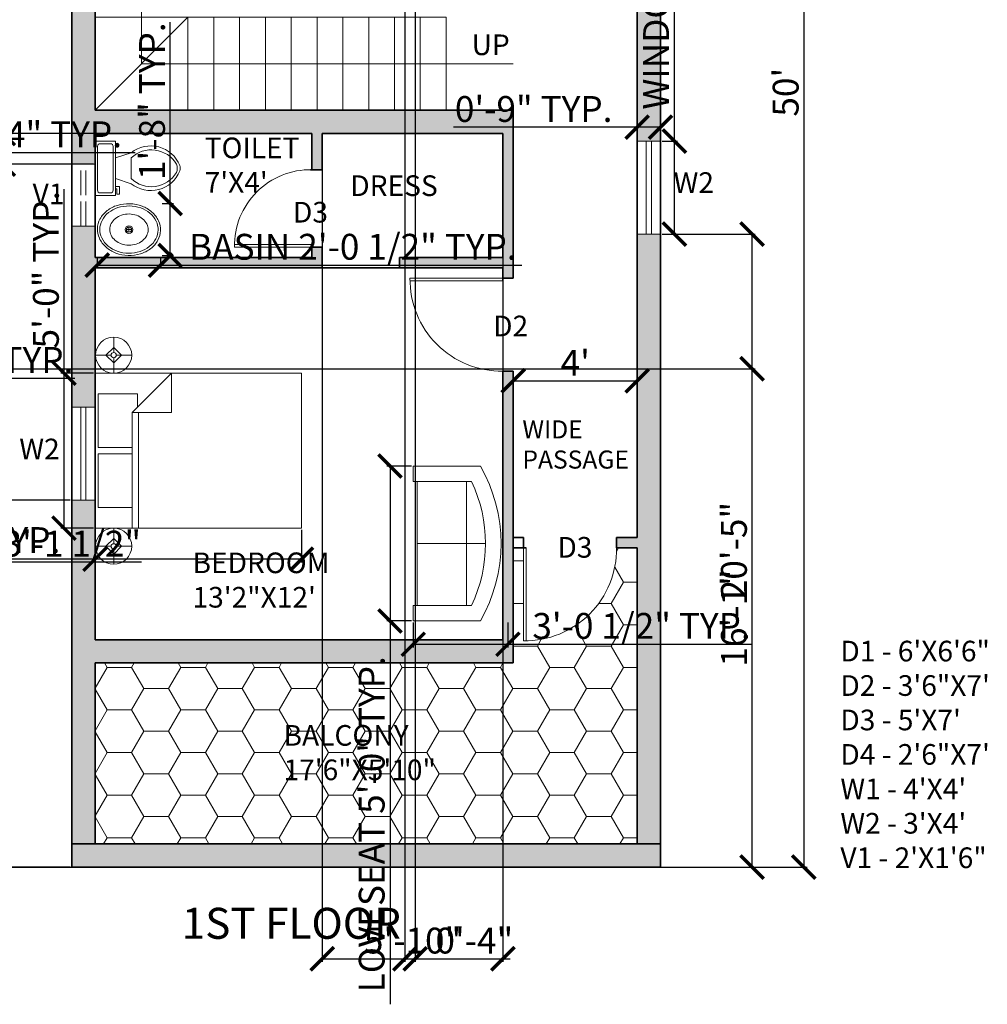
# Model space of a CAD drawing. Units: inches. Extents: x 2570 to 3313, y 1387 to 2106.
# Tile 4 of 5: x 2938 to 3313, y 1387 to 1769. Entities that reach past the tile are written whole.
import ezdxf

# ---------------------------------------------------------------- set-up
doc = ezdxf.new("R2010")
doc.units = ezdxf.units.IN
doc.linetypes.add('ACAD_ISO02W100', pattern=[15, 12, -3])
for name, color, linetype, lineweight in [('A-ANNO-DIMS', 7, 'Continuous', 18), ('A-ANNO-SYMB', 13, 'Continuous', 13), ('bed', 221, 'Continuous', 18), ('DOORS', 195, 'Continuous', 18), ('furniture', 11, 'Continuous', 18), ('P-FIXT', 8, 'Continuous', 18), ('STAIRS', 13, 'Continuous', 18), ('VENTILATORS', 143, 'ACAD_ISO02W100', 18), ('WALLS', 20, 'Continuous', 35), ('WINDOWS', 15, 'Continuous', 18)]:
    doc.layers.add(name, color=color, linetype=linetype, lineweight=lineweight)
for name, color, linetype, lineweight, true_color in [('A-ANNO-TEXT', 143, 'Continuous', 18, 0x7aafdf), ('A-ANNO-TITL', 52, 'Continuous', 25, 0xc8c92d), ('A-AREA-IDEN', 143, 'Continuous', 18, 0x7aafdf), ('A-FLOR-PATT', 254, 'Continuous', 13, 0xcecce6), ('A-WALL-PATT', 30, 'Continuous', 13, 0xf26722)]:
    doc.layers.add(name, color=color, linetype=linetype, lineweight=lineweight, true_color=true_color)
doc.styles.get("Standard").update_dxf_attribs({"font": 'arial.ttf'})
doc.dimstyles.new('ISO-25', dxfattribs={"dimtxt": 10, "dimasz": 9, "dimexe": 1.25, "dimexo": 0.625, "dimtad": 1, "dimdec": 0, "dimlunit": 3, "dimtxsty": 'Standard', "dimblk": 'ARCHTICK', "dimcen": 2.5, "dimadec": 0, "dimazin": 0, "dimtfac": 1, "dimtdec": 0, "dimtmove": 0, "dimatfit": 3, "dimfxl": 1, "dimarcsym": 0})

# ---------------------------------------------------------------- blocks, each defined once
blk = doc.blocks.new('Lamp - Table')
for p, q in [((0, 7), (0, 1)), ((-1, 0), (-7, 0)), ((0, 3), (-3, 0)), ((-3, 0), (0, -3)), ((3, 0), (0, 3)), ((0, -3), (3, 0)), ((1, 0), (7, 0)), ((0, -1), (0, -7))]:
    blk.add_line(p, q)
for radius in [7, 1]:
    blk.add_circle((0, 0), radius)
blk = doc.blocks.new('Bed - Queen')
for p, q in [((0, -80.00003), (0, 0)), ((0, 0), (59.99999, 0)), ((59.99999, 0), (59.99999, -80.00003)), ((7.99999, -1.2), (28.79998, -1.2)), ((7.99999, -14.4), (7.99999, -1.2)), ((28.79998, -1.2), (28.79998, -14.4)), ((31.19999, -1.2), (51.99999, -1.2)), ((31.19999, -14.4), (31.19999, -1.2)), ((51.99999, -1.2), (51.99999, -16.4)), ((0, -14.4), (44.8, -14.4)), ((59.99999, -29.6), (44.8, -14.4)), ((44.8, -14.4), (44.8, -29.6)), ((44.8, -16.8), (0, -16.8)), ((51.99999, -16.4), (46.79936, -16.4)), ((44.8, -29.6), (59.99999, -29.6)), ((59.99999, -80.00003), (0, -80.00003))]:
    blk.add_line(p, q)
blk = doc.blocks.new('Toilet - top')
for p, q in [((9.5, -6), (9.5, -2)), ((-10, -8.5), (-8, -8.5)), ((-10, -9.5), (-10, -8.5)), ((-7, -9.5), (-10, -9.5)), ((-8, -8.5), (-8, -8)), ((-7, -8), (-7, -9.5)), ((-4, -8), (-6, -14)), ((4, -8), (6, -14)), ((4, -14), (-4, -14))]:
    blk.add_line(p, q)
blk.add_lwpolyline([(10.5, -8), (10.5, 0), (-10.5, 0), (-10.5, -8)], close=True)
for points in [[(-9.5, -2), (-9.5, -6)], [(8.5, -1), (-8.5, -1)], [(-8.5, -7), (8.5, -7)]]:
    blk.add_lwpolyline(points)
for centre, radius, start, end in [((-8.62, -1.88), 0.884, 81.8699, 188.1301), ((8.62, -1.88), 0.884, 351.8699, 98.1301), ((-8.62, -6.12), 0.884, 171.8699, 278.1301), ((8.62, -6.12), 0.884, 261.8699, 8.1301), ((3.52, -21.58), 12.17, 141.4691, 247.9714), ((4.2, -21.82), 11.33, 136.3677, 238.9468), ((-3.52, -21.58), 12.17, 292.0284, 38.5307), ((-4.2, -21.82), 11.33, 301.053, 43.6321), ((0, -27.88), 4, 245.7318, 294.2682), ((0, -29), 4, 254.8605, 285.1395)]:
    blk.add_arc(centre, radius, start, end)
blk = doc.blocks.new('Sofa - Roundback Loveseat 5 ft.')
for p, q in [((0, -32.44198), (0, -5.99998)), ((-24, -33.99998), (-24, -11.46958)), ((-23.9998, -13.38178), (23.99986, -13.38178)), ((24.00004, -33.99998), (24.00004, -11.46958)), ((-24, -32.44198), (24.00004, -32.44198))]:
    blk.add_line(p, q)
for points in [[(-24, -33.99998), (-30, -33.99998), (-30, -7.99998)], [(30.00004, -7.99998), (30.00004, -33.99998), (24.00004, -33.99998)]]:
    blk.add_lwpolyline(points)
for centre, radius, start, end in [((0, -60.24998), 60.24998, 60.13715, 119.8628), ((0, -61.38438), 55.38444, 64.32083, 115.6792)]:
    blk.add_arc(centre, radius, start, end)
blk = doc.blocks.new('Sink - Oval top')
for p, q in [((-1, 0), (1, 0)), ((0, 1), (0, -1))]:
    blk.add_line(p, q)
for points in [[(-12.23, 0.39, 0.117634), (-11.46, -3.36, 0.104469), (-8.88, -6.8, 0.090016), (-5.08, -9.07, 0.08192), (-0.32, -10.02, 0.08192), (4.49, -9.38, 0.090016), (8.42, -7.36, 0.104469), (11.22, -4.09, 0.117634), (12.23, -0.39, 0.117634), (11.46, 3.36, 0.104469), (8.88, 6.8, 0.090016), (5.08, 9.07, 0.08192), (0.32, 10.02, 0.08192), (-4.49, 9.38, 0.090016), (-8.42, 7.36, 0.104469), (-11.22, 4.09, 0.117634)], [(-11.29, 0.16, 0.118622), (-10.52, -3.25, 0.104678), (-8.07, -6.36, 0.089562), (-4.54, -8.37, 0.081185), (-0.13, -9.15, 0.081185), (4.3, -8.49, 0.089562), (7.89, -6.58, 0.104678), (10.42, -3.55, 0.118622), (11.29, -0.16, 0.118622), (10.52, 3.25, 0.104678), (8.07, 6.36, 0.089562), (4.54, 8.37, 0.081185), (0.13, 9.15, 0.081185), (-4.3, 8.49, 0.089562), (-7.89, 6.58, 0.104678), (-10.42, 3.55, 0.118622)], [(-7.42, 0.08, 0.118283), (-6.91, -2.17, 0.104607), (-5.29, -4.21, 0.089718), (-2.97, -5.53, 0.081436), (-0.07, -6.04, 0.081436), (2.84, -5.59, 0.089718), (5.2, -4.33, 0.104607), (6.86, -2.32, 0.118283), (7.42, -0.08, 0.118283), (6.91, 2.17, 0.104607), (5.29, 4.21, 0.089718), (2.97, 5.53, 0.081436), (0.07, 6.04, 0.081436), (-2.84, 5.59, 0.089718), (-5.2, 4.33, 0.104607), (-6.86, 2.32, 0.118283)]]:
    blk.add_lwpolyline(points, format="xyb", close=True)
for radius in [1.5, 1]:
    blk.add_circle((0, 0), radius)
blk = doc.blocks.new('_ArchTick')
at = {"color": 0, "linetype": 'ByBlock', "const_width": 0.15}
blk.add_lwpolyline([(-0.5, -0.5), (0.5, 0.5)], dxfattribs=at)
blk = doc.blocks.new('*D19')
at = {"layer": 'A-ANNO-DIMS', "color": 0, "lineweight": -2, "transparency": 16777216}
for p, q in [((3186.79, 2040.49), (3242.94, 2040.49)), ((3241.69, 2040.49), (3241.69, 1440.49)), ((3186.79, 1440.49), (3242.94, 1440.49))]:
    blk.add_line(p, q, dxfattribs=at)
at = {"layer": 'Defpoints', "color": 0, "transparency": 16777216}
for p in [(3186.16, 2040.49), (3186.16, 1440.49), (3241.69, 1440.49)]:
    blk.add_point(p, dxfattribs=at)
at = {"layer": 'A-ANNO-DIMS', "color": 0, "lineweight": -2, "transparency": 16777216, "xscale": 9, "yscale": 9, "zscale": 9}
for p, rotation in [((3241.69, 2040.49), 90), ((3241.69, 1440.49), 270)]:
    blk.add_blockref('_ArchTick', p, dxfattribs=dict(at, rotation=rotation))
at = {"layer": 'A-ANNO-DIMS', "color": 0, "transparency": 16777216, "insert": (3235.96, 1740.49), "char_height": 10, "attachment_point": 5, "rotation": 90}
blk.add_mtext("50'", dxfattribs=at)
blk = doc.blocks.new('*D23')
at = {"layer": 'A-ANNO-DIMS', "color": 0, "lineweight": -2, "transparency": 16777216}
for p, q in [((3129.16, 1631.86), (3129.16, 1627.51)), ((3177.16, 1631.86), (3177.16, 1627.51)), ((3129.16, 1628.76), (3177.16, 1628.76))]:
    blk.add_line(p, q, dxfattribs=at)
at = {"layer": 'Defpoints', "color": 0, "transparency": 16777216}
for p in [(3129.16, 1632.49), (3177.16, 1632.49), (3177.16, 1628.76)]:
    blk.add_point(p, dxfattribs=at)
at = {"layer": 'A-ANNO-DIMS', "color": 0, "lineweight": -2, "transparency": 16777216, "xscale": 9, "yscale": 9, "zscale": 9, "rotation": 180}
blk.add_blockref('_ArchTick', (3129.16, 1628.76), dxfattribs=at)
at = {"layer": 'A-ANNO-DIMS', "color": 0, "lineweight": -2, "transparency": 16777216, "xscale": 9, "yscale": 9, "zscale": 9}
blk.add_blockref('_ArchTick', (3177.16, 1628.76), dxfattribs=at)
at = {"layer": 'A-ANNO-DIMS', "color": 0, "transparency": 16777216, "insert": (3153.16, 1634.38), "char_height": 10, "attachment_point": 5}
blk.add_mtext("4'", dxfattribs=at)
blk = doc.blocks.new('DOOR-SWING-30IN')
for p, q in [((0, 0), (-30, 0)), ((0, -1), (-30, -1))]:
    blk.add_line(p, q)
blk.add_arc((-0.5, -0.5), 29.5, 179.029, 270.971)
blk = doc.blocks.new('DOOR-SWING-36IN')
for p, q in [((-1, 0), (-1, 36)), ((0, 0), (0, 36))]:
    blk.add_line(p, q)
blk.add_arc((-0.5, 0.5), 35.5, 89.1931, 180.8069)
blk = doc.blocks.new('WIN-36IN')
for p, q in [((-36, 0), (-36, 9)), ((0, 0), (0, 9)), ((-36, 5.5), (0, 5.5)), ((-36, 3.5), (0, 3.5))]:
    blk.add_line(p, q)
blk = doc.blocks.new('VENT-V1-24IN')
for p, q in [((0, 0), (9, 0)), ((0, -24), (9, -24))]:
    blk.add_line(p, q)
at = {"ltscale": 0.8}
for p, q in [((3.5, -24), (3.5, 0)), ((5.5, -24), (5.5, 0))]:
    blk.add_line(p, q, dxfattribs=at)
blk = doc.blocks.new('STAIR-FLIGHT-36IN-WINDER')
for p, q in [((136, 36), (0, 36)), ((36, 36), (0, 0)), ((36, 0), (36, 36)), ((46, 0), (46, 36)), ((56, 0), (56, 36)), ((66, 0), (66, 36)), ((76, 0), (76, 36)), ((86, 0), (86, 36)), ((96, 0), (96, 36)), ((106, 0), (106, 36)), ((116, 0), (116, 36)), ((126, 0), (126, 36)), ((136, 0), (136, 36))]:
    blk.add_line(p, q)
blk = doc.blocks.new('*D35')
at = {"layer": 'A-ANNO-DIMS', "color": 0, "lineweight": -2, "transparency": 16777216}
for p, q in [((3191.56, 1721.56), (3191.56, 1858.35)), ((3186.79, 1721.56), (3192.81, 1721.56)), ((3191.56, 1685.56), (3191.56, 1721.56)), ((3186.79, 1685.56), (3192.81, 1685.56))]:
    blk.add_line(p, q, dxfattribs=at)
at = {"layer": 'Defpoints', "color": 0, "transparency": 16777216}
for p in [(3186.16, 1721.56), (3191.56, 1721.56), (3186.16, 1685.56)]:
    blk.add_point(p, dxfattribs=at)
at = {"layer": 'A-ANNO-DIMS', "color": 0, "lineweight": -2, "transparency": 16777216, "xscale": 9, "yscale": 9, "zscale": 9}
for p, rotation in [((3191.56, 1721.56), 90), ((3191.56, 1685.56), 270)]:
    blk.add_blockref('_ArchTick', p, dxfattribs=dict(at, rotation=rotation))
at = {"layer": 'A-ANNO-DIMS', "color": 0, "transparency": 16777216, "insert": (3185.76, 1794.46), "char_height": 10, "attachment_point": 5, "rotation": 90}
blk.add_mtext('WINDOW 3\'-0" TYP.', dxfattribs=at)
blk = doc.blocks.new('*D36')
at = {"layer": 'A-ANNO-DIMS', "color": 0, "lineweight": -2, "transparency": 16777216}
for p, q in [((3177.16, 1726.96), (3105.96, 1726.96)), ((3177.16, 1722.19), (3177.16, 1728.21)), ((3186.16, 1726.96), (3177.16, 1726.96)), ((3186.16, 1722.19), (3186.16, 1728.21))]:
    blk.add_line(p, q, dxfattribs=at)
at = {"layer": 'Defpoints', "color": 0, "transparency": 16777216}
for p in [(3177.16, 1726.96), (3177.16, 1721.56), (3186.16, 1721.56)]:
    blk.add_point(p, dxfattribs=at)
at = {"layer": 'A-ANNO-DIMS', "color": 0, "lineweight": -2, "transparency": 16777216, "xscale": 9, "yscale": 9, "zscale": 9}
for p, rotation in [((3177.16, 1726.96), 180.0000000000029), ((3186.16, 1726.96), 2.8777e-12)]:
    blk.add_blockref('_ArchTick', p, dxfattribs=dict(at, rotation=rotation))
at = {"layer": 'A-ANNO-DIMS', "color": 0, "transparency": 16777216, "insert": (3137.06, 1732.69), "char_height": 10, "attachment_point": 5}
blk.add_mtext('0\'-9" TYP.', dxfattribs=at)
blk = doc.blocks.new('*D44')
at = {"layer": 'A-ANNO-DIMS', "color": 0, "lineweight": -2, "transparency": 16777216}
for p, q in [((2879.15, 1632.78), (2879.15, 1628.55)), ((2888.15, 1632.78), (2888.15, 1628.55)), ((2879.15, 1629.8), (2888.15, 1629.8)), ((2888.15, 1629.8), (2959.36, 1629.8))]:
    blk.add_line(p, q, dxfattribs=at)
at = {"layer": 'Defpoints', "color": 0, "transparency": 16777216}
for p in [(2879.15, 1633.4), (2888.15, 1633.4), (2888.15, 1629.8)]:
    blk.add_point(p, dxfattribs=at)
at = {"layer": 'A-ANNO-DIMS', "color": 0, "lineweight": -2, "transparency": 16777216, "xscale": 9, "yscale": 9, "zscale": 9, "rotation": 180}
blk.add_blockref('_ArchTick', (2879.15, 1629.8), dxfattribs=at)
at = {"layer": 'A-ANNO-DIMS', "color": 0, "lineweight": -2, "transparency": 16777216, "xscale": 9, "yscale": 9, "zscale": 9}
blk.add_blockref('_ArchTick', (2888.15, 1629.8), dxfattribs=at)
at = {"layer": 'A-ANNO-DIMS', "color": 0, "transparency": 16777216, "insert": (2928.26, 1635.53), "char_height": 10, "attachment_point": 5}
blk.add_mtext('0\'-9" TYP.', dxfattribs=at)
blk = doc.blocks.new('*D45')
at = {"layer": 'A-ANNO-DIMS', "color": 0, "lineweight": -2, "transparency": 16777216}
for p, q in [((3089.8, 1595.75), (3080.17, 1595.75)), ((3081.42, 1595.75), (3081.42, 1535.75)), ((3089.8, 1535.75), (3080.17, 1535.75)), ((3081.42, 1535.75), (3081.42, 1387.35))]:
    blk.add_line(p, q, dxfattribs=at)
at = {"layer": 'Defpoints', "color": 0, "transparency": 16777216}
for p in [(3090.42, 1595.75), (3081.42, 1535.75), (3090.42, 1535.75)]:
    blk.add_point(p, dxfattribs=at)
at = {"layer": 'A-ANNO-DIMS', "color": 0, "lineweight": -2, "transparency": 16777216, "xscale": 9, "yscale": 9, "zscale": 9}
for p, rotation in [((3081.42, 1595.75), 90), ((3081.42, 1535.75), 270)]:
    blk.add_blockref('_ArchTick', p, dxfattribs=dict(at, rotation=rotation))
at = {"layer": 'A-ANNO-DIMS', "color": 0, "transparency": 16777216, "insert": (3075.62, 1457.05), "char_height": 10, "attachment_point": 5, "rotation": 90}
blk.add_mtext('LOVESEAT 5\'-0" TYP.', dxfattribs=at)
blk = doc.blocks.new('*D46')
at = {"layer": 'A-ANNO-DIMS', "color": 0, "lineweight": -2, "transparency": 16777216}
for p, q in [((3090.42, 1535.12), (3090.42, 1525.5)), ((3127.09, 1535.12), (3127.09, 1525.5)), ((3090.42, 1526.75), (3127.09, 1526.75)), ((3127.09, 1526.75), (3221.59, 1526.75))]:
    blk.add_line(p, q, dxfattribs=at)
at = {"layer": 'Defpoints', "color": 0, "transparency": 16777216}
for p in [(3090.42, 1535.75), (3127.09, 1535.75), (3127.09, 1526.75)]:
    blk.add_point(p, dxfattribs=at)
at = {"layer": 'A-ANNO-DIMS', "color": 0, "lineweight": -2, "transparency": 16777216, "xscale": 9, "yscale": 9, "zscale": 9, "rotation": 180}
blk.add_blockref('_ArchTick', (3090.42, 1526.75), dxfattribs=at)
at = {"layer": 'A-ANNO-DIMS', "color": 0, "lineweight": -2, "transparency": 16777216, "xscale": 9, "yscale": 9, "zscale": 9}
blk.add_blockref('_ArchTick', (3127.09, 1526.75), dxfattribs=at)
at = {"layer": 'A-ANNO-DIMS', "color": 0, "transparency": 16777216, "insert": (3178.84, 1532.55), "char_height": 10, "attachment_point": 5}
blk.add_mtext('3\'-0 1/2" TYP.', dxfattribs=at)
blk = doc.blocks.new('*D49')
at = {"layer": 'A-ANNO-DIMS', "color": 0, "lineweight": -2, "transparency": 16777216}
for p, q in [((2967.16, 1571.06), (2967.16, 1558.44)), ((3047.16, 1571.06), (3047.16, 1558.44)), ((2967.16, 1559.69), (2809.81, 1559.69)), ((3047.16, 1559.69), (2967.16, 1559.69))]:
    blk.add_line(p, q, dxfattribs=at)
at = {"layer": 'Defpoints', "color": 0, "transparency": 16777216}
for p in [(2967.16, 1571.69), (3047.16, 1571.69), (2967.16, 1559.69)]:
    blk.add_point(p, dxfattribs=at)
at = {"layer": 'A-ANNO-DIMS', "color": 0, "lineweight": -2, "transparency": 16777216, "xscale": 9, "yscale": 9, "zscale": 9, "rotation": 180}
blk.add_blockref('_ArchTick', (2967.16, 1559.69), dxfattribs=at)
at = {"layer": 'A-ANNO-DIMS', "color": 0, "lineweight": -2, "transparency": 16777216, "xscale": 9, "yscale": 9, "zscale": 9}
blk.add_blockref('_ArchTick', (3047.16, 1559.69), dxfattribs=at)
at = {"layer": 'A-ANNO-DIMS', "color": 0, "transparency": 16777216, "insert": (2883.99, 1565.79), "char_height": 10, "attachment_point": 5}
blk.add_mtext('QUEEN BED 6\'-8" TYP.', dxfattribs=at)
blk = doc.blocks.new('*D50')
at = {"layer": 'A-ANNO-DIMS', "color": 0, "lineweight": -2, "transparency": 16777216}
for p, q in [((2955.16, 1631.69), (2955.16, 1702.89)), ((2966.54, 1631.69), (2953.91, 1631.69)), ((2955.16, 1571.69), (2955.16, 1631.69)), ((2966.54, 1571.69), (2953.91, 1571.69))]:
    blk.add_line(p, q, dxfattribs=at)
at = {"layer": 'Defpoints', "color": 0, "transparency": 16777216}
for p in [(2955.16, 1631.69), (2967.16, 1631.69), (2967.16, 1571.69)]:
    blk.add_point(p, dxfattribs=at)
at = {"layer": 'A-ANNO-DIMS', "color": 0, "lineweight": -2, "transparency": 16777216, "xscale": 9, "yscale": 9, "zscale": 9}
for p, rotation in [((2955.16, 1631.69), 90), ((2955.16, 1571.69), 270)]:
    blk.add_blockref('_ArchTick', p, dxfattribs=dict(at, rotation=rotation))
at = {"layer": 'A-ANNO-DIMS', "color": 0, "transparency": 16777216, "insert": (2949.43, 1671.79), "char_height": 10, "attachment_point": 5, "rotation": 90}
blk.add_mtext('5\'-0" TYP.', dxfattribs=at)
blk = doc.blocks.new('*D51')
at = {"layer": 'A-ANNO-DIMS', "color": 0, "lineweight": -2, "transparency": 16777216}
for p, q in [((2968.04, 1676.6), (2968.04, 1672.29)), ((2968.04, 1673.54), (2992.59, 1673.54)), ((2992.59, 1676.6), (2992.59, 1672.29)), ((2992.59, 1673.54), (3132.46, 1673.54))]:
    blk.add_line(p, q, dxfattribs=at)
at = {"layer": 'Defpoints', "color": 0, "transparency": 16777216}
for p in [(2968.04, 1677.23), (2992.59, 1677.23), (2992.59, 1673.54)]:
    blk.add_point(p, dxfattribs=at)
at = {"layer": 'A-ANNO-DIMS', "color": 0, "lineweight": -2, "transparency": 16777216, "xscale": 9, "yscale": 9, "zscale": 9, "rotation": 180}
blk.add_blockref('_ArchTick', (2968.04, 1673.54), dxfattribs=at)
at = {"layer": 'A-ANNO-DIMS', "color": 0, "lineweight": -2, "transparency": 16777216, "xscale": 9, "yscale": 9, "zscale": 9}
blk.add_blockref('_ArchTick', (2992.59, 1673.54), dxfattribs=at)
at = {"layer": 'A-ANNO-DIMS', "color": 0, "transparency": 16777216, "insert": (3067.02, 1679.34), "char_height": 10, "attachment_point": 5}
blk.add_mtext('BASIN 2\'-0 1/2" TYP.', dxfattribs=at)
blk = doc.blocks.new('*D52')
at = {"layer": 'A-ANNO-DIMS', "color": 0, "lineweight": -2, "transparency": 16777216}
for p, q in [((2996.27, 1697.36), (2996.27, 1767.63)), ((2993.21, 1697.36), (2997.52, 1697.36)), ((2996.27, 1677.23), (2996.27, 1697.36)), ((2993.21, 1677.23), (2997.52, 1677.23))]:
    blk.add_line(p, q, dxfattribs=at)
at = {"layer": 'Defpoints', "color": 0, "transparency": 16777216}
for p in [(2992.59, 1697.36), (2996.27, 1697.36), (2992.59, 1677.23)]:
    blk.add_point(p, dxfattribs=at)
at = {"layer": 'A-ANNO-DIMS', "color": 0, "lineweight": -2, "transparency": 16777216, "xscale": 9, "yscale": 9, "zscale": 9}
for p, rotation in [((2996.27, 1697.36), 90), ((2996.27, 1677.23), 270)]:
    blk.add_blockref('_ArchTick', p, dxfattribs=dict(at, rotation=rotation))
at = {"layer": 'A-ANNO-DIMS', "color": 0, "transparency": 16777216, "insert": (2990.54, 1736.99), "char_height": 10, "attachment_point": 5, "rotation": 90}
blk.add_mtext('1\'-8" TYP.', dxfattribs=at)
blk = doc.blocks.new('*D53')
at = {"layer": 'A-ANNO-DIMS', "color": 0, "lineweight": -2, "transparency": 16777216}
for p, q in [((2669.15, 1736.86), (2669.15, 1715.84)), ((2805.15, 1736.86), (2805.15, 1715.84)), ((2669.15, 1717.09), (2805.15, 1717.09)), ((2805.15, 1717.09), (2982.66, 1717.09))]:
    blk.add_line(p, q, dxfattribs=at)
at = {"layer": 'Defpoints', "color": 0, "transparency": 16777216}
for p in [(2669.15, 1737.49), (2805.15, 1737.49), (2805.15, 1717.09)]:
    blk.add_point(p, dxfattribs=at)
at = {"layer": 'A-ANNO-DIMS', "color": 0, "lineweight": -2, "transparency": 16777216, "xscale": 9, "yscale": 9, "zscale": 9, "rotation": 180}
blk.add_blockref('_ArchTick', (2669.15, 1717.09), dxfattribs=at)
at = {"layer": 'A-ANNO-DIMS', "color": 0, "lineweight": -2, "transparency": 16777216, "xscale": 9, "yscale": 9, "zscale": 9}
blk.add_blockref('_ArchTick', (2805.15, 1717.09), dxfattribs=at)
at = {"layer": 'A-ANNO-DIMS', "color": 0, "transparency": 16777216, "insert": (2898.41, 1722.88), "char_height": 10, "attachment_point": 5}
blk.add_mtext('STAIR FLIGHT 11\'-4" TYP.', dxfattribs=at)
blk = doc.blocks.new('*D55')
at = {"layer": 'A-ANNO-DIMS', "color": 0, "lineweight": -2, "transparency": 16777216}
for p, q in [((2839.28, 1563.6), (2839.28, 1557.37)), ((2876.67, 1563.6), (2876.67, 1557.37)), ((2839.28, 1558.62), (2876.67, 1558.62)), ((2876.67, 1558.62), (2985.22, 1558.62))]:
    blk.add_line(p, q, dxfattribs=at)
at = {"layer": 'Defpoints', "color": 0, "transparency": 16777216}
for p in [(2839.28, 1564.23), (2876.67, 1564.23), (2876.67, 1558.62)]:
    blk.add_point(p, dxfattribs=at)
at = {"layer": 'A-ANNO-DIMS', "color": 0, "lineweight": -2, "transparency": 16777216, "xscale": 9, "yscale": 9, "zscale": 9, "rotation": 180}
blk.add_blockref('_ArchTick', (2839.28, 1558.62), dxfattribs=at)
at = {"layer": 'A-ANNO-DIMS', "color": 0, "lineweight": -2, "transparency": 16777216, "xscale": 9, "yscale": 9, "zscale": 9}
blk.add_blockref('_ArchTick', (2876.67, 1558.62), dxfattribs=at)
at = {"layer": 'A-ANNO-DIMS', "color": 0, "transparency": 16777216, "insert": (2935.45, 1564.42), "char_height": 10, "attachment_point": 5}
blk.add_mtext('PLANT 3\'-1 1/2"', dxfattribs=at)
blk = doc.blocks.new('*D63')
at = {"layer": 'A-ANNO-DIMS', "color": 0, "lineweight": -2, "transparency": 16777216}
for p, q in [((3055.16, 1723.86), (3055.16, 1403.74)), ((3125.16, 1723.86), (3125.16, 1403.74)), ((3055.16, 1404.99), (3125.16, 1404.99))]:
    blk.add_line(p, q, dxfattribs=at)
at = {"layer": 'Defpoints', "color": 0, "transparency": 16777216}
for p in [(3055.16, 1724.49), (3125.16, 1724.49), (3125.16, 1404.99)]:
    blk.add_point(p, dxfattribs=at)
at = {"layer": 'A-ANNO-DIMS', "color": 0, "lineweight": -2, "transparency": 16777216, "xscale": 9, "yscale": 9, "zscale": 9, "rotation": 180}
blk.add_blockref('_ArchTick', (3055.16, 1404.99), dxfattribs=at)
at = {"layer": 'A-ANNO-DIMS', "color": 0, "lineweight": -2, "transparency": 16777216, "xscale": 9, "yscale": 9, "zscale": 9}
blk.add_blockref('_ArchTick', (3125.16, 1404.99), dxfattribs=at)
at = {"layer": 'A-ANNO-DIMS', "color": 0, "transparency": 16777216, "insert": (3090.16, 1410.72), "char_height": 10, "attachment_point": 5}
blk.add_mtext('5\'-10"', dxfattribs=at)
blk = doc.blocks.new('*D69')
at = {"layer": 'A-ANNO-DIMS', "color": 0, "lineweight": -2, "transparency": 16777216}
for p, q in [((2957.54, 1582.49), (2623.4, 1582.49)), ((2624.65, 1440.49), (2624.65, 1582.49)), ((2957.54, 1440.49), (2623.4, 1440.49))]:
    blk.add_line(p, q, dxfattribs=at)
at = {"layer": 'Defpoints', "color": 0, "transparency": 16777216}
for p in [(2624.65, 1582.49), (2958.16, 1582.49), (2958.16, 1440.49)]:
    blk.add_point(p, dxfattribs=at)
at = {"layer": 'A-ANNO-DIMS', "color": 0, "lineweight": -2, "transparency": 16777216, "xscale": 9, "yscale": 9, "zscale": 9}
for p, rotation in [((2624.65, 1582.49), 90), ((2624.65, 1440.49), 270)]:
    blk.add_blockref('_ArchTick', p, dxfattribs=dict(at, rotation=rotation))
at = {"layer": 'A-ANNO-DIMS', "color": 0, "transparency": 16777216, "insert": (2618.92, 1511.49), "char_height": 10, "attachment_point": 5, "rotation": 90}
blk.add_mtext('11\'-10"', dxfattribs=at)
blk = doc.blocks.new('*D71')
at = {"layer": 'A-ANNO-DIMS', "color": 0, "lineweight": -2, "transparency": 16777216}
for p, q in [((3186.79, 1685.56), (3222.91, 1685.56)), ((3221.66, 1440.49), (3221.66, 1685.56)), ((3186.79, 1440.49), (3222.91, 1440.49))]:
    blk.add_line(p, q, dxfattribs=at)
at = {"layer": 'Defpoints', "color": 0, "transparency": 16777216}
for p in [(3186.16, 1685.56), (3221.66, 1685.56), (3186.16, 1440.49)]:
    blk.add_point(p, dxfattribs=at)
at = {"layer": 'A-ANNO-DIMS', "color": 0, "lineweight": -2, "transparency": 16777216, "xscale": 9, "yscale": 9, "zscale": 9}
for p, rotation in [((3221.66, 1685.56), 90), ((3221.66, 1440.49), 270)]:
    blk.add_blockref('_ArchTick', p, dxfattribs=dict(at, rotation=rotation))
at = {"layer": 'A-ANNO-DIMS', "color": 0, "transparency": 16777216, "insert": (3215.93, 1563.02), "char_height": 10, "attachment_point": 5, "rotation": 90}
blk.add_mtext('20\'-5"', dxfattribs=at)
blk = doc.blocks.new('*D76')
at = {"layer": 'A-ANNO-DIMS', "color": 0, "lineweight": -2, "transparency": 16777216}
for p, q in [((2888.78, 1633.4), (3222.91, 1633.4)), ((3221.66, 1440.49), (3221.66, 1633.4)), ((2888.78, 1440.49), (3222.91, 1440.49))]:
    blk.add_line(p, q, dxfattribs=at)
at = {"layer": 'Defpoints', "color": 0, "transparency": 16777216}
for p in [(2888.15, 1633.4), (3221.66, 1633.4), (2888.15, 1440.49)]:
    blk.add_point(p, dxfattribs=at)
at = {"layer": 'A-ANNO-DIMS', "color": 0, "lineweight": -2, "transparency": 16777216, "xscale": 9, "yscale": 9, "zscale": 9}
for p, rotation in [((3221.66, 1633.4), 90), ((3221.66, 1440.49), 270)]:
    blk.add_blockref('_ArchTick', p, dxfattribs=dict(at, rotation=rotation))
at = {"layer": 'A-ANNO-DIMS', "color": 0, "transparency": 16777216, "insert": (3215.93, 1536.94), "char_height": 10, "attachment_point": 5, "rotation": 90}
blk.add_mtext('16\'-1"', dxfattribs=at)
blk = doc.blocks.new('*D77')
at = {"layer": 'A-ANNO-DIMS', "color": 0, "lineweight": -2, "transparency": 16777216}
for p, q in [((2931.66, 1724.49), (2931.66, 1760.38)), ((2966.54, 1724.49), (2930.41, 1724.49)), ((2931.66, 1712.62), (2931.66, 1724.49)), ((2966.54, 1712.62), (2930.41, 1712.62))]:
    blk.add_line(p, q, dxfattribs=at)
at = {"layer": 'Defpoints', "color": 0, "transparency": 16777216}
for p in [(2931.66, 1724.49), (2967.16, 1724.49), (2967.16, 1712.62)]:
    blk.add_point(p, dxfattribs=at)
at = {"layer": 'A-ANNO-DIMS', "color": 0, "lineweight": -2, "transparency": 16777216, "xscale": 9, "yscale": 9, "zscale": 9}
for p, rotation in [((2931.66, 1724.49), 90), ((2931.66, 1712.62), 270)]:
    blk.add_blockref('_ArchTick', p, dxfattribs=dict(at, rotation=rotation))
at = {"layer": 'A-ANNO-DIMS', "color": 0, "transparency": 16777216, "insert": (2925.93, 1746.93), "char_height": 10, "attachment_point": 5, "rotation": 90}
blk.add_mtext('1\'-0"', dxfattribs=at)
blk = doc.blocks.new('*D79')
at = {"layer": 'A-ANNO-DIMS', "color": 0, "lineweight": -2, "transparency": 16777216}
for p, q in [((3087.16, 2030.86), (3087.16, 1403.74)), ((3091.16, 2030.86), (3091.16, 1403.74)), ((3087.16, 1404.99), (3091.16, 1404.99)), ((3091.16, 1404.99), (3128, 1404.99))]:
    blk.add_line(p, q, dxfattribs=at)
at = {"layer": 'Defpoints', "color": 0, "transparency": 16777216}
for p in [(3087.16, 2031.49), (3091.16, 2031.49), (3091.16, 1404.99)]:
    blk.add_point(p, dxfattribs=at)
at = {"layer": 'A-ANNO-DIMS', "color": 0, "lineweight": -2, "transparency": 16777216, "xscale": 9, "yscale": 9, "zscale": 9, "rotation": 180}
blk.add_blockref('_ArchTick', (3087.16, 1404.99), dxfattribs=at)
at = {"layer": 'A-ANNO-DIMS', "color": 0, "lineweight": -2, "transparency": 16777216, "xscale": 9, "yscale": 9, "zscale": 9}
blk.add_blockref('_ArchTick', (3091.16, 1404.99), dxfattribs=at)
at = {"layer": 'A-ANNO-DIMS', "color": 0, "transparency": 16777216, "insert": (3114.08, 1410.72), "char_height": 10, "attachment_point": 5}
blk.add_mtext('0\'-4"', dxfattribs=at)

msp = doc.modelspace()

# ---------------------------------------------------------------- hatches: boundary and pattern name
at = {"layer": 'A-FLOR-PATT'}
h = msp.add_hatch(dxfattribs=at)
h.set_pattern_fill('HONEY', color=256, scale=3)
h.paths.add_polyline_path([(3177.16, 1519.49), (3177.16, 1564.09), (3169.16, 1564.09, -0.422488), (3133.16, 1528.09), (3133.16, 1564.09), (3129.16, 1564.09), (3129.16, 1519.49), (2967.16, 1519.49), (2967.16, 1449.49), (3177.16, 1449.49)])
at = {"layer": 'A-WALL-PATT'}
h = msp.add_hatch(color=256, dxfattribs=at)
h.dxf.hatch_style = 1
h.paths.add_polyline_path([(2888.15, 1871.99), (2879.15, 1871.99), (2879.15, 1817.49), (2851.15, 1817.49), (2851.15, 1813.49), (2879.15, 1813.49), (2879.15, 1657.4), (2888.15, 1657.4)])
h.paths.add_polyline_path([(2831.15, 1737.49), (2669.15, 1737.49), (2669.15, 1813.49), (2745.15, 1813.49), (2745.15, 1849.49), (2741.15, 1849.49), (2741.15, 1817.49), (2669.15, 1817.49), (2669.15, 1838.62), (2660.15, 1838.62), (2660.15, 1669.99), (2669.15, 1669.99), (2669.15, 1728.49), (2831.15, 1728.49)])
h.paths.add_polyline_path([(2669.15, 1621.99), (2660.15, 1621.99), (2660.15, 1440.49), (2802.65, 1440.49), (2802.65, 1449.49), (2669.15, 1449.49), (2669.15, 1554.49), (2700.9, 1554.49), (2700.9, 1563.49), (2669.15, 1563.49)])
h.paths.add_polyline_path([(2780.65, 1563.49), (2748.9, 1563.49), (2748.9, 1554.49), (2780.65, 1554.49)], flags=17)
h.paths.add_polyline_path([(2836.15, 1599.49), (2879.15, 1599.49), (2879.15, 1449.49), (2874.65, 1449.49), (2874.65, 1440.49), (2888.15, 1440.49), (2888.15, 1633.4), (2879.15, 1633.4), (2879.15, 1608.49), (2831.15, 1608.49), (2831.15, 1680.49), (2827.15, 1680.49), (2827.15, 1563.49), (2822.65, 1563.49), (2822.65, 1554.49), (2836.15, 1554.49)])
h.paths.add_polyline_path([(2793.15, 1962.49), (2821.15, 1962.49), (2821.15, 1971.49), (2793.15, 1971.49), (2793.15, 2031.49), (2818.15, 2031.49), (2818.15, 2040.49), (2747.15, 2040.49), (2747.15, 2031.49), (2789.15, 2031.49), (2789.15, 1887.49), (2785.15, 1887.49), (2785.15, 1879.49), (2789.15, 1879.49), (2789.15, 1817.49), (2789.15, 1813.49), (2793.15, 1813.49), (2821.15, 1813.49), (2821.15, 1817.49), (2793.15, 1817.49)])
h.paths.add_polyline_path([(2749.15, 1887.49), (2669.15, 1887.49), (2669.15, 2031.49), (2711.15, 2031.49), (2711.15, 2040.49), (2660.15, 2040.49), (2660.15, 1862.62), (2669.15, 1862.62), (2669.15, 1883.49), (2741.15, 1883.49), (2741.15, 1879.49), (2749.15, 1879.49)])
h.paths.add_polyline_path([(2888.15, 2040.49), (2854.15, 2040.49), (2854.15, 2031.49), (2879.15, 2031.49), (2879.15, 1971.49), (2877.15, 1971.49), (2877.15, 1962.49), (2879.15, 1962.49), (2879.15, 1907.99), (2888.15, 1907.99)])
h.paths.add_polyline_path([(2967.16, 2031.49), (3011.16, 2031.49), (3011.16, 2004.49), (3015.16, 2004.49), (3015.16, 2031.49), (3039.26, 2031.49), (3039.26, 2040.49), (2958.16, 2040.49), (2958.16, 1909.99), (2967.16, 1909.99), (2967.16, 1921.99), (2967.16, 1966.49)])
h.paths.add_polyline_path([(3186.16, 2040.49), (3063.26, 2040.49), (3063.26, 2031.49), (3087.16, 2031.49), (3087.16, 1970.49), (3015.16, 1970.49), (3015.16, 1974.49), (3011.16, 1974.49), (3011.16, 1966.49), (3177.16, 1966.49), (3177.16, 1817.49), (3172.66, 1817.49), (3172.66, 1813.49), (3177.16, 1813.49), (3177.16, 1721.56), (3186.16, 1721.56)])
h.paths.add_polyline_path([(3177.16, 2031.49), (3177.16, 1970.49), (3091.16, 1970.49), (3091.16, 2031.49)], flags=16)
h.paths.add_polyline_path([(2967.16, 1873.99), (2958.16, 1873.99), (2958.16, 1712.62), (2967.16, 1712.62), (2967.16, 1724.49), (3051.16, 1724.49), (3051.16, 1710.49), (3055.16, 1710.49), (3055.16, 1724.49), (3125.16, 1724.49), (3125.16, 1676.49), (3085.16, 1676.49), (3085.16, 1672.49), (3125.16, 1672.49), (3125.16, 1668.49), (3129.16, 1668.49), (3129.16, 1733.49), (2967.16, 1733.49), (2967.16, 1813.49), (3136.66, 1813.49), (3136.66, 1817.49), (2967.16, 1817.49)])
h.paths.add_polyline_path([(2967.16, 1672.49), (3055.16, 1672.49), (3055.16, 1680.49), (3051.16, 1680.49), (3051.16, 1676.49), (2967.16, 1676.49), (2967.16, 1688.62), (2958.16, 1688.62), (2958.16, 1618.49), (2967.16, 1618.49), (2967.16, 1631.69)])
h.paths.add_polyline_path([(3186.16, 1685.56), (3177.16, 1685.56), (3177.16, 1568.09), (3169.16, 1568.09), (3169.16, 1564.09), (3177.16, 1564.09), (3177.16, 1519.49), (3177.16, 1449.49), (3186.16, 1449.49)])
h.paths.add_polyline_path([(3129.16, 1564.09), (3129.16, 1632.49), (3125.16, 1632.49), (3125.16, 1528.49), (2967.16, 1528.49), (2967.16, 1582.49), (2958.16, 1582.49), (2958.16, 1449.49), (2967.16, 1449.49), (2967.16, 1519.49), (3129.16, 1519.49)])
h.paths.add_polyline_path([(3123.16, 1975.63), (3150.13, 1975.63), (3150.13, 1992.12), (3123.16, 1992.12)], flags=8)
h.paths.add_polyline_path([(3130.18, 1590.82), (3180.42, 1590.82), (3180.42, 1617.03), (3130.18, 1617.03)], flags=9)
h = msp.add_hatch(color=256, dxfattribs=at)
h.dxf.hatch_style = 1
h.paths.add_polyline_path([(3186.16, 1449.49), (2958.16, 1449.49), (2958.16, 1440.49), (3186.16, 1440.49)])

# ---------------------------------------------------------------- linework, layer by layer
at = {"layer": 'A-ANNO-SYMB'}
for p, q in [((2985.16, 1751.49), (2985.16, 1773.49)), ((3129.16, 1751.49), (2985.16, 1751.49))]:
    msp.add_line(p, q, dxfattribs=at)
at = {"layer": 'WALLS'}
for p, q in [((2958.16, 2040.49), (2958.16, 1440.49)), ((3186.16, 1440.49), (3186.16, 2040.49)), ((2967.16, 1813.49), (2967.16, 1733.49)), ((3177.16, 1568.09), (3177.16, 1813.49)), ((2967.16, 1733.49), (3129.16, 1733.49)), ((3129.16, 1733.49), (3129.16, 1668.49)), ((2967.16, 1724.49), (3051.16, 1724.49)), ((2967.16, 1724.49), (2967.16, 1676.49)), ((3051.16, 1724.49), (3051.16, 1710.49)), ((3055.16, 1724.49), (3055.16, 1710.49)), ((3055.16, 1724.49), (3125.16, 1724.49)), ((3125.16, 1724.49), (3125.16, 1676.49)), ((3050.66, 1710.49), (3055.16, 1710.49)), ((3051.16, 1681.49), (3051.16, 1676.49)), ((3051.16, 1680.49), (3055.16, 1680.49)), ((3055.16, 1680.49), (3055.16, 1672.49)), ((2967.16, 1676.49), (3051.16, 1676.49)), ((3085.16, 1676.49), (3125.16, 1676.49)), ((3085.16, 1676.49), (3085.16, 1672.49)), ((2967.16, 1672.49), (3125.16, 1672.49)), ((2967.16, 1672.49), (2967.16, 1528.49)), ((3125.16, 1672.49), (3125.16, 1667.49)), ((3125.16, 1668.49), (3129.16, 1668.49)), ((3125.16, 1632.49), (3129.16, 1632.49)), ((3125.16, 1632.49), (3125.16, 1528.49)), ((3129.16, 1632.49), (3129.16, 1564.09)), ((3129.16, 1568.09), (3133.16, 1568.09)), ((3133.16, 1568.09), (3133.16, 1564.09)), ((3169.16, 1568.09), (3169.16, 1564.09)), ((3169.16, 1568.09), (3177.16, 1568.09)), ((3129.16, 1564.09), (3134.16, 1564.09)), ((3129.16, 1564.09), (3129.16, 1519.49)), ((3169.16, 1564.09), (3177.16, 1564.09)), ((3177.16, 1519.49), (3177.16, 1564.09)), ((2967.16, 1528.49), (3125.16, 1528.49)), ((2967.16, 1519.49), (3129.16, 1519.49)), ((2967.16, 1519.49), (2967.16, 1449.49)), ((3177.16, 1449.49), (3177.16, 1519.49)), ((2958.16, 1449.49), (3186.16, 1449.49)), ((2958.16, 1440.49), (3186.16, 1440.49))]:
    msp.add_line(p, q, dxfattribs=at)

# ---------------------------------------------------------------- block references
at = {"layer": 'bed', "xscale": -1, "rotation": 180}
msp.add_blockref('Lamp - Table', (2974.39, 1638.68), dxfattribs=at)
at = {"layer": 'bed', "rotation": 90}
msp.add_blockref('Bed - Queen', (2967.16, 1571.69), dxfattribs=at)
at = {"layer": 'bed'}
msp.add_blockref('Lamp - Table', (2974.39, 1564.69), dxfattribs=at)
at = {"layer": 'DOORS', "extrusion": (0, 0, -1), "zscale": -1, "rotation": 180}
msp.add_blockref('DOOR-SWING-30IN', (-3051.16, 1680.49), dxfattribs=at)
at = {"layer": 'DOORS'}
for p, rotation in [((3125.16, 1668.49), 89.99999999998796), ((3133.16, 1564.09), 180)]:
    msp.add_blockref('DOOR-SWING-36IN', p, dxfattribs=dict(at, rotation=rotation))
at = {"layer": 'furniture', "rotation": 270}
msp.add_blockref('Sofa - Roundback Loveseat 5 ft.', (3124.42, 1565.75), dxfattribs=at)
at = {"layer": 'P-FIXT', "rotation": 89.99999999999999}
msp.add_blockref('Toilet - top', (2967.16, 1711.03), dxfattribs=at)
at = {"layer": 'P-FIXT'}
msp.add_blockref('Sink - Oval top', (2980.31, 1687.29), dxfattribs=at)
at = {"layer": 'STAIRS'}
msp.add_blockref('STAIR-FLIGHT-36IN-WINDER', (2967.16, 1733.49), dxfattribs=at)
at = {"layer": 'VENTILATORS'}
msp.add_blockref('VENT-V1-24IN', (2958.16, 1712.62), dxfattribs=at)
at = {"layer": 'WINDOWS'}
for p, rotation in [((3186.16, 1721.56), 90.00000000000273), ((2967.16, 1618.49), 89.99999999999967)]:
    msp.add_blockref('WIN-36IN', p, dxfattribs=dict(at, rotation=rotation))

# ---------------------------------------------------------------- texts
at = {"layer": 'A-ANNO-TEXT', "char_height": 8, "attachment_point": 1}
for s, width, insert in [('UP', 60.8198, (3113.03, 1762.84)), ('W2', 13.4987, (3191.26, 1709.49)), ('V1', 13.4987, (2942.98, 1705.13)), ('D3', 13.0839, (3043.83, 1698.02)), ('D2', 13.0839, (3121.37, 1653.96)), ('W2', 13.4987, (2937.84, 1606.34)), ('D3', 13.0839, (3146.26, 1568.27)), ('D1 - 6\'X6\'6"\\PD2 - 3\'6"X7\'\\PD3 - 5\'X7\'\\PD4 - 2\'6"X7\'\\PW1 - 4\'X4\'\\PW2 - 3\'X4\'\\PV1 - 2\'X1\'6"\\P ', 579.7175, (3255.85, 1528.1))]:
    msp.add_mtext_dynamic_manual_height_columns(s, width=width, gutter_width=12.5, heights=[0], dxfattribs=dict(at, insert=insert))
at = {"layer": 'A-ANNO-TITL', "insert": (3000.75, 1424.7), "char_height": 12, "attachment_point": 1}
msp.add_mtext_dynamic_manual_height_columns('{\\fArial|b1|i0|c0|p34;1ST FLOOR}', width=181.3713, gutter_width=12.5, heights=[0], dxfattribs=at)
at = {"layer": 'A-AREA-IDEN', "attachment_point": 1}
for s, insert, char_height in [("TOILET\\P7'X4'", (3009.63, 1722.92), 8), ('DRESS', (3066.03, 1708.29), 8), ('WIDE PASSAGE', (3132.69, 1613.43), 7), ('BEDROOM\\P13\'2"X12\'', (3004.92, 1562.27), 8), ('BALCONY\\P17\'6"X5\'10"', (3040.17, 1495.46), 8)]:
    msp.add_mtext_dynamic_manual_height_columns(s, width=60.8198, gutter_width=12.5, heights=[0], dxfattribs=dict(at, insert=insert, char_height=char_height))

# ---------------------------------------------------------------- dimensions: what is measured, and where the dimension line sits
at = {"layer": 'A-ANNO-DIMS'}
for base, p1, p2, override, picture, middle in [((3241.69, 1440.49), (3186.16, 2040.49), (3186.16, 1440.49), {"dimclrd": 0, "dimclre": 0, "dimclrt": 0}, '*D19', (3235.96, 1740.49)), ((2931.66, 1724.49), (2967.16, 1712.62), (2967.16, 1724.49), {"dimdec": 1, "dimlfac": 1, "dimrnd": 0, "dimzin": 1, "dimdsep": 46, "dimlunit": 4, "dimfrac": 2}, '*D77', (2925.93, 1746.93)), ((3221.66, 1685.56), (3186.16, 1440.49), (3186.16, 1685.56), {"dimdec": 1, "dimlfac": 1, "dimrnd": 0, "dimzin": 1, "dimdsep": 46, "dimlunit": 4, "dimfrac": 2}, '*D71', (3215.93, 1563.02)), ((3221.66, 1633.4), (2888.15, 1440.49), (2888.15, 1633.4), {"dimdec": 1, "dimlfac": 1, "dimrnd": 0, "dimzin": 1, "dimdsep": 46, "dimlunit": 4, "dimfrac": 2}, '*D76', (3215.93, 1536.94)), ((2624.65, 1582.49), (2958.16, 1440.49), (2958.16, 1582.49), {"dimdec": 1, "dimlfac": 1, "dimrnd": 0, "dimzin": 1, "dimdsep": 46, "dimlunit": 4, "dimfrac": 2}, '*D69', (2618.92, 1511.49))]:
    dim = msp.add_linear_dim(base=base, p1=p1, p2=p2, angle=90, dimstyle='ISO-25', override=override, dxfattribs=at)
    dim.commit()
    dim.dimension.update_dxf_attribs({"geometry": picture, "text_midpoint": middle})
for base, p1, p2, override, picture, middle in [((3091.16, 1404.99), (3087.16, 2031.49), (3091.16, 2031.49), {"dimdec": 1, "dimlfac": 1, "dimrnd": 0, "dimzin": 1, "dimdsep": 46, "dimlunit": 4, "dimfrac": 2}, '*D79', (3114.08, 1410.72)), ((3125.16, 1404.99), (3055.16, 1724.49), (3125.16, 1724.49), {"dimdec": 1, "dimlfac": 1, "dimrnd": 0, "dimzin": 1, "dimdsep": 46, "dimlunit": 4, "dimfrac": 2}, '*D63', (3090.16, 1410.72)), ((3177.16, 1628.76), (3129.16, 1632.49), (3177.16, 1632.49), {"dimclrd": 0, "dimclre": 0, "dimclrt": 0}, '*D23', (3153.16, 1634.38))]:
    dim = msp.add_linear_dim(base=base, p1=p1, p2=p2, dimstyle='ISO-25', override=override, dxfattribs=at)
    dim.commit()
    dim.dimension.update_dxf_attribs({"geometry": picture, "text_midpoint": middle})
for base, p1, p2, angle, text, picture, middle in [((3191.56, 1721.56), (3186.16, 1685.56), (3186.16, 1721.56), 90, 'WINDOW <> TYP.', '*D35', (3185.76, 1794.46)), ((2996.27, 1697.36), (2992.59, 1677.23), (2992.59, 1697.36), 90, '<> TYP.', '*D52', (2990.54, 1736.99)), ((3177.16, 1726.96), (3186.16, 1721.56), (3177.16, 1721.56), 180, '<> TYP.', '*D36', (3137.06, 1732.69)), ((2955.16, 1631.69), (2967.16, 1571.69), (2967.16, 1631.69), 90, '<> TYP.', '*D50', (2949.43, 1671.79)), ((2967.16, 1559.69), (3047.16, 1571.69), (2967.16, 1571.69), 180, 'QUEEN BED <> TYP.', '*D49', (2883.99, 1565.79)), ((3081.42, 1535.75), (3090.42, 1595.75), (3090.42, 1535.75), 270, 'LOVESEAT <> TYP.', '*D45', (3075.62, 1457.05))]:
    dim = msp.add_linear_dim(base=base, p1=p1, p2=p2, angle=angle, text=text, dimstyle='ISO-25', override={"dimdec": 1, "dimlfac": 1, "dimrnd": 0, "dimzin": 1, "dimdsep": 46, "dimlunit": 4, "dimfrac": 2}, dxfattribs=at)
    dim.commit()
    dim.dimension.update_dxf_attribs({"geometry": picture, "text_midpoint": middle})
for base, p1, p2, text, picture, middle in [((2805.15, 1717.09), (2669.15, 1737.49), (2805.15, 1737.49), 'STAIR FLIGHT <> TYP.', '*D53', (2898.41, 1722.88)), ((2992.5879, 1673.543), (2968.037, 1677.2256), (2992.5879, 1677.2256), 'BASIN <> TYP.', '*D51', (3067.0219, 1679.3385)), ((2888.15, 1629.8), (2879.15, 1633.4), (2888.15, 1633.4), '<> TYP.', '*D44', (2928.26, 1635.53)), ((2876.67, 1558.62), (2839.28, 1564.23), (2876.67, 1564.23), 'PLANT <>', '*D55', (2935.45, 1564.42)), ((3127.09, 1526.75), (3090.42, 1535.75), (3127.09, 1535.75), '<> TYP.', '*D46', (3178.84, 1532.55))]:
    dim = msp.add_linear_dim(base=base, p1=p1, p2=p2, text=text, dimstyle='ISO-25', override={"dimdec": 1, "dimlfac": 1, "dimrnd": 0, "dimzin": 1, "dimdsep": 46, "dimlunit": 4, "dimfrac": 2}, dxfattribs=at)
    dim.commit()
    dim.dimension.update_dxf_attribs({"geometry": picture, "text_midpoint": middle})

doc.saveas('drawing.dxf')
